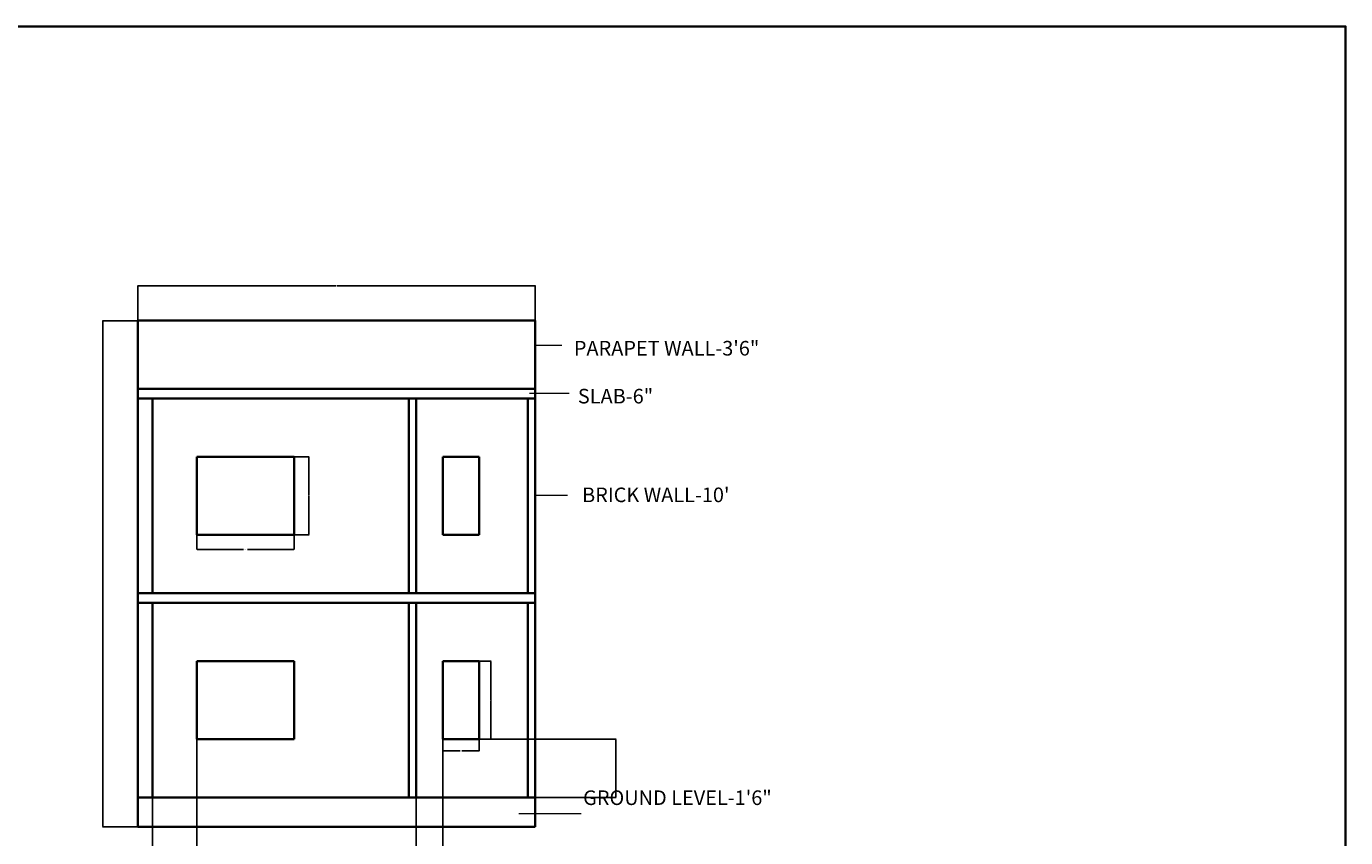
# Model space of a CAD drawing. Units: inches. Extents: x 1850 to 3445, y 1558 to 2756.
# Tile 13 of 13: x 2632 to 3445, y 2256 to 2756. Entities that reach past the tile are written whole.
import ezdxf

# ---------------------------------------------------------------- set-up
doc = ezdxf.new("R2010")
doc.units = ezdxf.units.IN
for name, color, linetype, lineweight in [('A-ANNO-DIMS', 2, 'Continuous', 18), ('A-ANNO-SYMB', 2, 'Continuous', 18), ('A-ANNO-TEXT', 7, 'Continuous', 18), ('A-ANNO-TTLB', 7, 'Continuous', 35), ('A-SECT', 7, 'Continuous', 35)]:
    doc.layers.add(name, color=color, linetype=linetype, lineweight=lineweight)
doc.styles.get("Standard").update_dxf_attribs({"font": 'arial.ttf'})
doc.dimstyles.get("Standard").update_dxf_attribs({"dimtxt": 0.18, "dimasz": 0.18, "dimexe": 0.18, "dimexo": 0.0625, "dimgap": 0.09, "dimtad": 0, "dimtih": 1, "dimtoh": 1, "dimdec": 4, "dimzin": 0, "dimdsep": 46, "dimtxsty": 'Standard', "dimcen": 0.09, "dimadec": 0, "dimazin": 0, "dimtfac": 1, "dimtdec": 4, "dimtofl": 0, "dimtmove": 0, "dimatfit": 3, "dimfxl": 1, "dimtolj": 1, "dimtzin": 0, "dimarcsym": 0})

# ---------------------------------------------------------------- blocks, each defined once
blk = doc.blocks.new('SECTION-OPENING-WIDE')
for p, q in [((0, 48), (0, 0)), ((60, 48), (0, 48)), ((60, 48), (60, 0)), ((60, 0), (0, 0))]:
    blk.add_line(p, q)
blk = doc.blocks.new('SECTION-OPENING-NARROW')
for p, q in [((0, 48), (0, 0)), ((22.27, 48), (0, 48)), ((22.27, 48), (22.27, 0)), ((22.27, 0), (0, 0))]:
    blk.add_line(p, q)
blk = doc.blocks.new('*D76')
at = {"layer": 'A-ANNO-DIMS', "color": 0, "lineweight": -2, "transparency": 16777216}
for p, q in [((2737.2, 2442.81), (2737.2, 2433.69)), ((2797.2, 2442.81), (2797.2, 2433.69)), ((2737.38, 2433.87), (2766.06, 2433.87)), ((2797.02, 2433.87), (2768.34, 2433.87))]:
    blk.add_line(p, q, dxfattribs=at)
at = {"layer": 'A-ANNO-DIMS', "color": 0, "transparency": 16777216}
for points in [[(2737.38, 2433.9), (2737.38, 2433.84), (2737.2, 2433.87)], [(2797.02, 2433.9), (2797.02, 2433.84), (2797.2, 2433.87)]]:
    blk.add_solid(points, dxfattribs=at)
at = {"layer": 'Defpoints', "color": 0, "transparency": 16777216}
for p in [(2737.2, 2442.87), (2797.2, 2442.87), (2797.2, 2433.87)]:
    blk.add_point(p, dxfattribs=at)
at = {"layer": 'A-ANNO-DIMS', "color": 0, "transparency": 16777216, "insert": (2767.2, 2433.87), "char_height": 0.18, "attachment_point": 5}
blk.add_mtext('\\A1;OPENING 60 TYP.', dxfattribs=at)
blk = doc.blocks.new('*D77')
at = {"layer": 'A-ANNO-DIMS', "color": 0, "lineweight": -2, "transparency": 16777216}
for p, q in [((2797.26, 2490.87), (2806.38, 2490.87)), ((2806.2, 2490.69), (2806.2, 2467.06)), ((2806.2, 2443.05), (2806.2, 2466.69)), ((2797.26, 2442.87), (2806.38, 2442.87))]:
    blk.add_line(p, q, dxfattribs=at)
at = {"layer": 'A-ANNO-DIMS', "color": 0, "transparency": 16777216}
for points in [[(2806.17, 2490.69), (2806.23, 2490.69), (2806.2, 2490.87)], [(2806.17, 2443.05), (2806.23, 2443.05), (2806.2, 2442.87)]]:
    blk.add_solid(points, dxfattribs=at)
at = {"layer": 'Defpoints', "color": 0, "transparency": 16777216}
for p in [(2797.2, 2490.87), (2806.2, 2490.87), (2797.2, 2442.87)]:
    blk.add_point(p, dxfattribs=at)
at = {"layer": 'A-ANNO-DIMS', "color": 0, "transparency": 16777216, "insert": (2806.2, 2466.87), "char_height": 0.18, "attachment_point": 5}
blk.add_mtext('\\A1;48 TYP.', dxfattribs=at)
blk = doc.blocks.new('*D78')
at = {"layer": 'A-ANNO-DIMS', "color": 0, "lineweight": -2, "transparency": 16777216}
for p, q in [((2911.23, 2364.87), (2918.55, 2364.87)), ((2918.37, 2364.69), (2918.37, 2341.06)), ((2918.37, 2317.05), (2918.37, 2340.69)), ((2911.23, 2316.87), (2918.55, 2316.87))]:
    blk.add_line(p, q, dxfattribs=at)
at = {"layer": 'A-ANNO-DIMS', "color": 0, "transparency": 16777216}
for points in [[(2918.34, 2364.69), (2918.4, 2364.69), (2918.37, 2364.87)], [(2918.34, 2317.05), (2918.4, 2317.05), (2918.37, 2316.87)]]:
    blk.add_solid(points, dxfattribs=at)
at = {"layer": 'Defpoints', "color": 0, "transparency": 16777216}
for p in [(2911.17, 2364.87), (2918.37, 2364.87), (2911.17, 2316.87)]:
    blk.add_point(p, dxfattribs=at)
at = {"layer": 'A-ANNO-DIMS', "color": 0, "transparency": 16777216, "insert": (2918.37, 2340.87), "char_height": 0.18, "attachment_point": 5}
blk.add_mtext('\\A1;OPENING 48 TYP.', dxfattribs=at)
blk = doc.blocks.new('*D79')
at = {"layer": 'A-ANNO-DIMS', "color": 0, "lineweight": -2, "transparency": 16777216}
for p, q in [((2888.9, 2316.81), (2888.9, 2309.49)), ((2889.08, 2309.67), (2899.5, 2309.67)), ((2910.99, 2309.67), (2900.56, 2309.67)), ((2911.17, 2316.81), (2911.17, 2309.49))]:
    blk.add_line(p, q, dxfattribs=at)
at = {"layer": 'A-ANNO-DIMS', "color": 0, "transparency": 16777216}
for points in [[(2889.08, 2309.7), (2889.08, 2309.64), (2888.9, 2309.67)], [(2910.99, 2309.7), (2910.99, 2309.64), (2911.17, 2309.67)]]:
    blk.add_solid(points, dxfattribs=at)
at = {"layer": 'Defpoints', "color": 0, "transparency": 16777216}
for p in [(2888.9, 2316.87), (2911.17, 2316.87), (2911.17, 2309.67)]:
    blk.add_point(p, dxfattribs=at)
at = {"layer": 'A-ANNO-DIMS', "color": 0, "transparency": 16777216, "insert": (2900.03, 2309.67), "char_height": 0.18, "attachment_point": 5}
blk.add_mtext('\\A1;22 TYP.', dxfattribs=at)
blk = doc.blocks.new('*D122')
at = {"layer": 'A-ANNO-DIMS', "color": 0, "lineweight": -2, "transparency": 16777216}
for p, q in [((2700.82, 2574.94), (2700.82, 2596.55)), ((2701, 2596.37), (2823.03, 2596.37)), ((2945.64, 2596.37), (2823.61, 2596.37)), ((2945.82, 2574.94), (2945.82, 2596.55))]:
    blk.add_line(p, q, dxfattribs=at)
at = {"layer": 'A-ANNO-DIMS', "color": 0, "transparency": 16777216}
for points in [[(2701, 2596.4), (2701, 2596.34), (2700.82, 2596.37)], [(2945.64, 2596.4), (2945.64, 2596.34), (2945.82, 2596.37)]]:
    blk.add_solid(points, dxfattribs=at)
at = {"layer": 'Defpoints', "color": 0, "transparency": 16777216}
for p in [(2945.82, 2596.37), (2700.82, 2574.87), (2945.82, 2574.87)]:
    blk.add_point(p, dxfattribs=at)
at = {"layer": 'A-ANNO-DIMS', "color": 0, "transparency": 16777216, "insert": (2823.32, 2596.37), "char_height": 0.18, "attachment_point": 5}
blk.add_mtext('\\A1;245', dxfattribs=at)
blk = doc.blocks.new('*D123')
at = {"layer": 'A-ANNO-DIMS', "color": 0, "lineweight": -2, "transparency": 16777216}
for p, q in [((2700.76, 2574.87), (2679.14, 2574.87)), ((2679.32, 2574.69), (2679.32, 2419.06)), ((2679.32, 2263.05), (2679.32, 2418.69)), ((2700.76, 2262.87), (2679.14, 2262.87))]:
    blk.add_line(p, q, dxfattribs=at)
at = {"layer": 'A-ANNO-DIMS', "color": 0, "transparency": 16777216}
for points in [[(2679.29, 2574.69), (2679.35, 2574.69), (2679.32, 2574.87)], [(2679.29, 2263.05), (2679.35, 2263.05), (2679.32, 2262.87)]]:
    blk.add_solid(points, dxfattribs=at)
at = {"layer": 'Defpoints', "color": 0, "transparency": 16777216}
for p in [(2679.32, 2574.87), (2700.82, 2574.87), (2700.82, 2262.87)]:
    blk.add_point(p, dxfattribs=at)
at = {"layer": 'A-ANNO-DIMS', "color": 0, "transparency": 16777216, "insert": (2679.32, 2418.87), "char_height": 0.18, "attachment_point": 5}
blk.add_mtext('\\A1;312', dxfattribs=at)
blk = doc.blocks.new('*D124')
at = {"layer": 'A-ANNO-DIMS', "color": 0, "lineweight": -2, "transparency": 16777216}
for p, q in [((2737.2, 2316.81), (2737.2, 2241.19)), ((2709.82, 2280.81), (2709.82, 2241.19)), ((2710, 2241.37), (2723.05, 2241.37)), ((2737.02, 2241.37), (2723.98, 2241.37))]:
    blk.add_line(p, q, dxfattribs=at)
at = {"layer": 'A-ANNO-DIMS', "color": 0, "transparency": 16777216}
for points in [[(2710, 2241.4), (2710, 2241.34), (2709.82, 2241.37)], [(2737.02, 2241.4), (2737.02, 2241.34), (2737.2, 2241.37)]]:
    blk.add_solid(points, dxfattribs=at)
at = {"layer": 'Defpoints', "color": 0, "transparency": 16777216}
for p in [(2737.2, 2316.87), (2709.82, 2280.87), (2737.2, 2241.37)]:
    blk.add_point(p, dxfattribs=at)
at = {"layer": 'A-ANNO-DIMS', "color": 0, "transparency": 16777216, "insert": (2723.51, 2241.37), "char_height": 0.18, "attachment_point": 5}
blk.add_mtext('\\A1;27.377', dxfattribs=at)
blk = doc.blocks.new('*D125')
at = {"layer": 'A-ANNO-DIMS', "color": 0, "lineweight": -2, "transparency": 16777216}
for p, q in [((2888.9, 2316.81), (2888.9, 2241.19)), ((2872.32, 2280.81), (2872.32, 2241.19)), ((2872.5, 2241.37), (2880.16, 2241.37)), ((2888.72, 2241.37), (2881.07, 2241.37))]:
    blk.add_line(p, q, dxfattribs=at)
at = {"layer": 'A-ANNO-DIMS', "color": 0, "transparency": 16777216}
for points in [[(2872.5, 2241.4), (2872.5, 2241.34), (2872.32, 2241.37)], [(2888.72, 2241.4), (2888.72, 2241.34), (2888.9, 2241.37)]]:
    blk.add_solid(points, dxfattribs=at)
at = {"layer": 'Defpoints', "color": 0, "transparency": 16777216}
for p in [(2888.9, 2316.87), (2872.32, 2280.87), (2888.9, 2241.37)]:
    blk.add_point(p, dxfattribs=at)
at = {"layer": 'A-ANNO-DIMS', "color": 0, "transparency": 16777216, "insert": (2880.61, 2241.37), "char_height": 0.18, "attachment_point": 5}
blk.add_mtext('\\A1;16.577', dxfattribs=at)
blk = doc.blocks.new('*D126')
at = {"layer": 'A-ANNO-DIMS', "color": 0, "lineweight": -2, "transparency": 16777216}
for p, q in [((2911.23, 2316.87), (2995.72, 2316.87)), ((2995.54, 2316.69), (2995.54, 2299.06)), ((2995.54, 2281.05), (2995.54, 2298.69)), ((2941.38, 2280.87), (2995.72, 2280.87))]:
    blk.add_line(p, q, dxfattribs=at)
at = {"layer": 'A-ANNO-DIMS', "color": 0, "transparency": 16777216}
for points in [[(2995.51, 2316.69), (2995.57, 2316.69), (2995.54, 2316.87)], [(2995.51, 2281.05), (2995.57, 2281.05), (2995.54, 2280.87)]]:
    blk.add_solid(points, dxfattribs=at)
at = {"layer": 'Defpoints', "color": 0, "transparency": 16777216}
for p in [(2911.17, 2316.87), (2995.54, 2316.87), (2941.32, 2280.87)]:
    blk.add_point(p, dxfattribs=at)
at = {"layer": 'A-ANNO-DIMS', "color": 0, "transparency": 16777216, "insert": (2995.54, 2298.87), "char_height": 0.18, "attachment_point": 5}
blk.add_mtext('\\A1;36', dxfattribs=at)

msp = doc.modelspace()

# ---------------------------------------------------------------- linework, layer by layer
at = {"layer": 'A-ANNO-SYMB'}
for p, q in [((2945.822, 2559.7901), (2962.127, 2559.7901)), ((2942.2402, 2530.1181), (2966.6877, 2530.1181)), ((2945.822, 2467.326), (2965.7196, 2467.326)), ((2935.739, 2270.9692), (2974.0402, 2270.9692))]:
    msp.add_line(p, q, dxfattribs=at)
at = {"layer": 'A-ANNO-TTLB'}
msp.add_lwpolyline([(1850.1793, 2756.3177), (3445.2682, 2756.3177), (3445.2682, 1557.7728), (1850.1793, 1557.7728)], close=True, dxfattribs=at)
at = {"layer": 'A-SECT'}
for p, q in [((2700.822, 2574.8737), (2700.822, 2388.8737)), ((2945.822, 2574.8737), (2700.822, 2574.8737)), ((2945.822, 2574.8737), (2945.822, 2388.8737)), ((2945.822, 2532.8737), (2700.822, 2532.8737)), ((2945.822, 2526.8737), (2700.822, 2526.8737)), ((2709.822, 2526.8737), (2709.822, 2406.8737)), ((2867.822, 2526.8737), (2867.822, 2406.8737)), ((2872.322, 2526.8737), (2872.322, 2406.8737)), ((2941.322, 2526.8737), (2941.322, 2406.8737)), ((2700.822, 2448.8737), (2700.822, 2262.8737)), ((2945.822, 2448.8737), (2945.822, 2262.8737)), ((2945.822, 2406.8737), (2700.822, 2406.8737)), ((2945.822, 2400.8737), (2700.822, 2400.8737)), ((2709.822, 2400.8737), (2709.822, 2280.8737)), ((2867.822, 2400.8737), (2867.822, 2280.8737)), ((2872.322, 2400.8737), (2872.322, 2280.8737)), ((2941.322, 2400.8737), (2941.322, 2280.8737)), ((2945.822, 2280.8737), (2700.822, 2280.8737)), ((2945.822, 2262.8737), (2700.822, 2262.8737))]:
    msp.add_line(p, q, dxfattribs=at)

# ---------------------------------------------------------------- block references
for name, p in [('SECTION-OPENING-WIDE', (2737.199, 2442.874)), ('SECTION-OPENING-NARROW', (2888.899, 2442.874)), ('SECTION-OPENING-WIDE', (2737.199, 2316.874)), ('SECTION-OPENING-NARROW', (2888.899, 2316.874))]:
    msp.add_blockref(name, p, dxfattribs=at)

# ---------------------------------------------------------------- texts
at = {"layer": 'A-ANNO-TEXT', "char_height": 9, "attachment_point": 1}
for s, width, insert in [('PARAPET WALL-3\'6"', 143.630651, (2969.5908, 2562.3866)), ('SLAB-6"', 41.118921, (2972.0655, 2532.8366)), ("BRICK WALL-10'", 100.489615, (2974.6675, 2471.9749)), ('GROUND LEVEL-1\'6"', 166.34743, (2975.287, 2285.2503))]:
    msp.add_mtext_dynamic_manual_height_columns(s, width=width, gutter_width=12.5, heights=[0], dxfattribs=dict(at, insert=insert))

# ---------------------------------------------------------------- dimensions: what is measured, and where the dimension line sits
at = {"layer": 'A-ANNO-DIMS'}
for base, p1, p2, override, picture, middle in [((2945.822, 2596.3737), (2700.822, 2574.8737), (2945.822, 2574.8737), {"dimdec": 0, "dimlfac": 1, "dimrnd": 0, "dimzin": 0, "dimdsep": 46, "dimlunit": 2}, '*D122', (2823.322, 2596.3737)), ((2737.1986, 2241.3737), (2709.822, 2280.8737), (2737.1986, 2316.8737), {"dimdec": 3, "dimlfac": 1, "dimrnd": 0, "dimzin": 0, "dimdsep": 46, "dimlunit": 2}, '*D124', (2723.5103, 2241.3737)), ((2888.8991, 2241.3737), (2872.322, 2280.8737), (2888.8991, 2316.8737), {"dimdec": 3, "dimlfac": 1, "dimrnd": 0, "dimzin": 0, "dimdsep": 46, "dimlunit": 2}, '*D125', (2880.6105, 2241.3737))]:
    dim = msp.add_linear_dim(base=base, p1=p1, p2=p2, dimstyle='Standard', override=override, dxfattribs=at)
    dim.commit()
    dim.dimension.update_dxf_attribs({"geometry": picture, "text_midpoint": middle})
for base, p1, p2, picture, middle in [((2679.322, 2574.8737), (2700.822, 2262.8737), (2700.822, 2574.8737), '*D123', (2679.322, 2418.8737)), ((2995.5402, 2316.8737), (2941.322, 2280.8737), (2911.1674, 2316.8737), '*D126', (2995.5402, 2298.8737))]:
    dim = msp.add_linear_dim(base=base, p1=p1, p2=p2, angle=90, dimstyle='Standard', override={"dimdec": 0, "dimlfac": 1, "dimrnd": 0, "dimzin": 0, "dimdsep": 46, "dimlunit": 2}, dxfattribs=at)
    dim.commit()
    dim.dimension.update_dxf_attribs({"geometry": picture, "text_midpoint": middle})
for base, p1, p2, text, picture, middle in [((2806.1986, 2490.8737), (2797.1986, 2442.8737), (2797.1986, 2490.8737), '<> TYP.', '*D77', (2806.1986, 2466.8737)), ((2918.3674, 2364.8737), (2911.1674, 2316.8737), (2911.1674, 2364.8737), 'OPENING <> TYP.', '*D78', (2918.3674, 2340.8737))]:
    dim = msp.add_linear_dim(base=base, p1=p1, p2=p2, angle=90, text=text, dimstyle='Standard', override={"dimdec": 0, "dimlfac": 1, "dimrnd": 0, "dimzin": 0, "dimdsep": 46, "dimlunit": 2}, dxfattribs=at)
    dim.commit()
    dim.dimension.update_dxf_attribs({"geometry": picture, "text_midpoint": middle})
for base, p1, p2, text, picture, middle in [((2797.1986, 2433.8737), (2737.1986, 2442.8737), (2797.1986, 2442.8737), 'OPENING <> TYP.', '*D76', (2767.1986, 2433.8737)), ((2911.1674, 2309.6737), (2888.8991, 2316.8737), (2911.1674, 2316.8737), '<> TYP.', '*D79', (2900.0332, 2309.6737))]:
    dim = msp.add_linear_dim(base=base, p1=p1, p2=p2, text=text, dimstyle='Standard', override={"dimdec": 0, "dimlfac": 1, "dimrnd": 0, "dimzin": 0, "dimdsep": 46, "dimlunit": 2}, dxfattribs=at)
    dim.commit()
    dim.dimension.update_dxf_attribs({"geometry": picture, "text_midpoint": middle})

doc.saveas('drawing.dxf')
